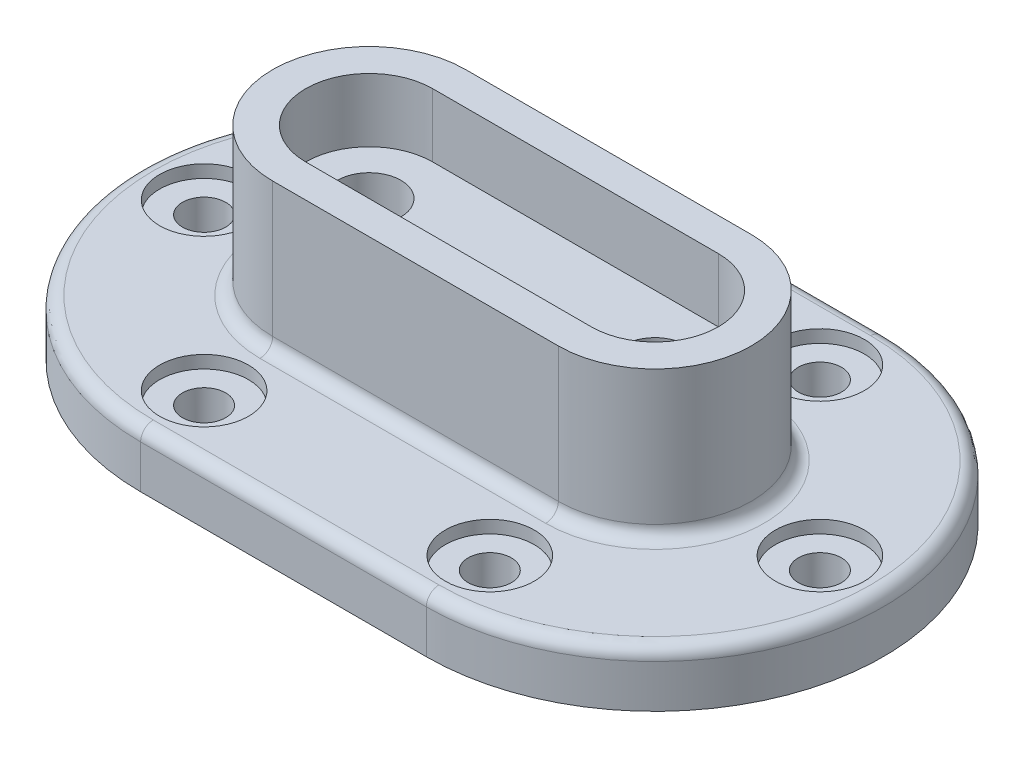
ISO-10303-21;
HEADER;
FILE_DESCRIPTION(('STEP AP214'),'2;1');
FILE_NAME('part.step','',(''),(''),'','','');
FILE_SCHEMA(('AUTOMOTIVE_DESIGN { 1 0 10303 214 1 1 1 1 }'));
ENDSEC;
DATA;
#1=APPLICATION_CONTEXT('core data for automotive mechanical design processes');
#2=APPLICATION_PROTOCOL_DEFINITION('international standard','automotive_design',2000,#1);
#3=PRODUCT_CONTEXT('',#1,'mechanical');
#4=PRODUCT('Part','Part','',(#3));
#5=PRODUCT_RELATED_PRODUCT_CATEGORY('part','',(#4));
#6=PRODUCT_DEFINITION_FORMATION('','',#4);
#7=PRODUCT_DEFINITION_CONTEXT('part definition',#1,'design');
#8=PRODUCT_DEFINITION('design','',#6,#7);
#9=PRODUCT_DEFINITION_SHAPE('','',#8);
#10=(LENGTH_UNIT() NAMED_UNIT(*) SI_UNIT(.MILLI.,.METRE.));
#11=(NAMED_UNIT(*) PLANE_ANGLE_UNIT() SI_UNIT($,.RADIAN.));
#12=(NAMED_UNIT(*) SI_UNIT($,.STERADIAN.) SOLID_ANGLE_UNIT());
#13=UNCERTAINTY_MEASURE_WITH_UNIT(LENGTH_MEASURE(1.E-05),#10,'distance_accuracy_value','');
#14=(GEOMETRIC_REPRESENTATION_CONTEXT(3) GLOBAL_UNCERTAINTY_ASSIGNED_CONTEXT((#13)) GLOBAL_UNIT_ASSIGNED_CONTEXT((#10,
#11,#12)) REPRESENTATION_CONTEXT('',''));
#15=CARTESIAN_POINT('',(0.,0.,0.));
#16=DIRECTION('',(0.,0.,1.));
#17=DIRECTION('',(1.,0.,0.));
#18=AXIS2_PLACEMENT_3D('',#15,#16,#17);
#19=CARTESIAN_POINT('',(11.25,4.4,0.));
#20=DIRECTION('',(0.,-1.,0.));
#21=DIRECTION('',(0.,0.,-1.));
#22=AXIS2_PLACEMENT_3D('',#19,#20,#21);
#23=CYLINDRICAL_SURFACE('',#22,18.);
#24=DIRECTION('',(0.,-1.,0.));
#25=VECTOR('',#24,1.);
#26=CARTESIAN_POINT('',(11.25,4.4,-18.));
#27=LINE('',#26,#25);
#28=CARTESIAN_POINT('',(11.25,3.4,-18.));
#29=VERTEX_POINT('',#28);
#30=CARTESIAN_POINT('',(11.25,0.,-18.));
#31=VERTEX_POINT('',#30);
#32=EDGE_CURVE('E243',#29,#31,#27,.T.);
#33=ORIENTED_EDGE('',*,*,#32,.F.);
#34=CARTESIAN_POINT('',(11.25,3.4,0.));
#35=DIRECTION('',(0.,1.,0.));
#36=DIRECTION('',(0.,0.,1.));
#37=AXIS2_PLACEMENT_3D('',#34,#35,#36);
#38=CIRCLE('',#37,18.);
#39=CARTESIAN_POINT('',(11.25,3.4,18.));
#40=VERTEX_POINT('',#39);
#41=EDGE_CURVE('E68',#29,#40,#38,.F.);
#42=ORIENTED_EDGE('',*,*,#41,.T.);
#43=DIRECTION('',(0.,-1.,0.));
#44=VECTOR('',#43,1.);
#45=CARTESIAN_POINT('',(11.25,4.4,18.));
#46=LINE('',#45,#44);
#47=CARTESIAN_POINT('',(11.25,0.,18.));
#48=VERTEX_POINT('',#47);
#49=EDGE_CURVE('E232',#40,#48,#46,.T.);
#50=ORIENTED_EDGE('',*,*,#49,.T.);
#51=CARTESIAN_POINT('',(11.25,0.,0.));
#52=DIRECTION('',(0.,1.,0.));
#53=DIRECTION('',(0.,0.,1.));
#54=AXIS2_PLACEMENT_3D('',#51,#52,#53);
#55=CIRCLE('',#54,18.);
#56=EDGE_CURVE('E224',#48,#31,#55,.T.);
#57=ORIENTED_EDGE('',*,*,#56,.T.);
#58=EDGE_LOOP('',(#33,#42,#50,#57));
#59=FACE_BOUND('',#58,.T.);
#60=ADVANCED_FACE('F41',(#59),#23,.T.);
#61=CARTESIAN_POINT('',(11.25,4.4,-18.));
#62=DIRECTION('',(0.,0.,1.));
#63=DIRECTION('',(1.,0.,0.));
#64=AXIS2_PLACEMENT_3D('',#61,#62,#63);
#65=PLANE('',#64);
#66=DIRECTION('',(0.,-1.,0.));
#67=VECTOR('',#66,1.);
#68=CARTESIAN_POINT('',(-11.25,4.4,-18.));
#69=LINE('',#68,#67);
#70=CARTESIAN_POINT('',(-11.25,3.4,-18.));
#71=VERTEX_POINT('',#70);
#72=CARTESIAN_POINT('',(-11.25,0.,-18.));
#73=VERTEX_POINT('',#72);
#74=EDGE_CURVE('E239',#71,#73,#69,.T.);
#75=ORIENTED_EDGE('',*,*,#74,.F.);
#76=DIRECTION('',(-1.,0.,0.));
#77=VECTOR('',#76,1.);
#78=CARTESIAN_POINT('',(11.25,3.4,-18.));
#79=LINE('',#78,#77);
#80=EDGE_CURVE('E286',#71,#29,#79,.F.);
#81=ORIENTED_EDGE('',*,*,#80,.T.);
#82=ORIENTED_EDGE('',*,*,#32,.T.);
#83=DIRECTION('',(-1.,0.,0.));
#84=VECTOR('',#83,1.);
#85=CARTESIAN_POINT('',(11.25,0.,-18.));
#86=LINE('',#85,#84);
#87=EDGE_CURVE('E228',#31,#73,#86,.T.);
#88=ORIENTED_EDGE('',*,*,#87,.T.);
#89=EDGE_LOOP('',(#75,#81,#82,#88));
#90=FACE_BOUND('',#89,.T.);
#91=ADVANCED_FACE('F328',(#90),#65,.F.);
#92=CARTESIAN_POINT('',(-11.25,4.4,0.));
#93=DIRECTION('',(0.,-1.,0.));
#94=DIRECTION('',(0.,0.,-1.));
#95=AXIS2_PLACEMENT_3D('',#92,#93,#94);
#96=CYLINDRICAL_SURFACE('',#95,18.);
#97=DIRECTION('',(0.,-1.,0.));
#98=VECTOR('',#97,1.);
#99=CARTESIAN_POINT('',(-11.25,4.4,18.));
#100=LINE('',#99,#98);
#101=CARTESIAN_POINT('',(-11.25,3.4,18.));
#102=VERTEX_POINT('',#101);
#103=CARTESIAN_POINT('',(-11.25,0.,18.));
#104=VERTEX_POINT('',#103);
#105=EDGE_CURVE('E240',#102,#104,#100,.T.);
#106=ORIENTED_EDGE('',*,*,#105,.F.);
#107=CARTESIAN_POINT('',(-11.25,3.4,0.));
#108=DIRECTION('',(0.,1.,0.));
#109=DIRECTION('',(0.,0.,1.));
#110=AXIS2_PLACEMENT_3D('',#107,#108,#109);
#111=CIRCLE('',#110,18.);
#112=EDGE_CURVE('E11',#102,#71,#111,.F.);
#113=ORIENTED_EDGE('',*,*,#112,.T.);
#114=ORIENTED_EDGE('',*,*,#74,.T.);
#115=CARTESIAN_POINT('',(-11.25,0.,0.));
#116=DIRECTION('',(0.,1.,0.));
#117=DIRECTION('',(0.,0.,1.));
#118=AXIS2_PLACEMENT_3D('',#115,#116,#117);
#119=CIRCLE('',#118,18.);
#120=EDGE_CURVE('E227',#73,#104,#119,.T.);
#121=ORIENTED_EDGE('',*,*,#120,.T.);
#122=EDGE_LOOP('',(#106,#113,#114,#121));
#123=FACE_BOUND('',#122,.T.);
#124=ADVANCED_FACE('F326',(#123),#96,.T.);
#125=CARTESIAN_POINT('',(11.25,4.4,18.));
#126=DIRECTION('',(0.,0.,-1.));
#127=DIRECTION('',(-1.,0.,0.));
#128=AXIS2_PLACEMENT_3D('',#125,#126,#127);
#129=PLANE('',#128);
#130=ORIENTED_EDGE('',*,*,#49,.F.);
#131=DIRECTION('',(1.,0.,0.));
#132=VECTOR('',#131,1.);
#133=CARTESIAN_POINT('',(-11.25,3.4,18.));
#134=LINE('',#133,#132);
#135=EDGE_CURVE('E59',#40,#102,#134,.F.);
#136=ORIENTED_EDGE('',*,*,#135,.T.);
#137=ORIENTED_EDGE('',*,*,#105,.T.);
#138=DIRECTION('',(1.,0.,0.));
#139=VECTOR('',#138,1.);
#140=CARTESIAN_POINT('',(11.25,0.,18.));
#141=LINE('',#140,#139);
#142=EDGE_CURVE('E235',#104,#48,#141,.T.);
#143=ORIENTED_EDGE('',*,*,#142,.T.);
#144=EDGE_LOOP('',(#130,#136,#137,#143));
#145=FACE_BOUND('',#144,.T.);
#146=ADVANCED_FACE('F339',(#145),#129,.F.);
#147=CARTESIAN_POINT('',(11.25,4.4,0.));
#148=DIRECTION('',(0.,1.,0.));
#149=DIRECTION('',(0.,0.,1.));
#150=AXIS2_PLACEMENT_3D('',#147,#148,#149);
#151=PLANE('',#150);
#152=CARTESIAN_POINT('',(-11.25,4.4,0.));
#153=DIRECTION('',(0.,1.,0.));
#154=DIRECTION('',(0.,0.,1.));
#155=AXIS2_PLACEMENT_3D('',#152,#153,#154);
#156=CIRCLE('',#155,8.6);
#157=CARTESIAN_POINT('',(-11.25,4.4,8.6));
#158=VERTEX_POINT('',#157);
#159=CARTESIAN_POINT('',(-11.25,4.4,-8.6));
#160=VERTEX_POINT('',#159);
#161=EDGE_CURVE('E274',#158,#160,#156,.F.);
#162=ORIENTED_EDGE('',*,*,#161,.T.);
#163=DIRECTION('',(-1.,0.,0.));
#164=VECTOR('',#163,1.);
#165=CARTESIAN_POINT('',(11.25,4.4,-8.6));
#166=LINE('',#165,#164);
#167=CARTESIAN_POINT('',(11.25,4.4,-8.6));
#168=VERTEX_POINT('',#167);
#169=EDGE_CURVE('E283',#160,#168,#166,.F.);
#170=ORIENTED_EDGE('',*,*,#169,.T.);
#171=CARTESIAN_POINT('',(11.25,4.4,0.));
#172=DIRECTION('',(0.,1.,0.));
#173=DIRECTION('',(0.,0.,1.));
#174=AXIS2_PLACEMENT_3D('',#171,#172,#173);
#175=CIRCLE('',#174,8.6);
#176=CARTESIAN_POINT('',(11.25,4.4,8.6));
#177=VERTEX_POINT('',#176);
#178=EDGE_CURVE('E276',#168,#177,#175,.F.);
#179=ORIENTED_EDGE('',*,*,#178,.T.);
#180=DIRECTION('',(1.,0.,0.));
#181=VECTOR('',#180,1.);
#182=CARTESIAN_POINT('',(11.25,4.4,8.6));
#183=LINE('',#182,#181);
#184=EDGE_CURVE('E280',#177,#158,#183,.F.);
#185=ORIENTED_EDGE('',*,*,#184,.T.);
#186=EDGE_LOOP('',(#162,#170,#179,#185));
#187=FACE_BOUND('',#186,.T.);
#188=CARTESIAN_POINT('',(11.25,4.4,0.));
#189=DIRECTION('',(0.,1.,0.));
#190=DIRECTION('',(0.,0.,1.));
#191=AXIS2_PLACEMENT_3D('',#188,#189,#190);
#192=CIRCLE('',#191,17.);
#193=CARTESIAN_POINT('',(11.25,4.4,17.));
#194=VERTEX_POINT('',#193);
#195=CARTESIAN_POINT('',(11.25,4.4,-17.));
#196=VERTEX_POINT('',#195);
#197=EDGE_CURVE('E269',#194,#196,#192,.T.);
#198=ORIENTED_EDGE('',*,*,#197,.T.);
#199=DIRECTION('',(-1.,0.,0.));
#200=VECTOR('',#199,1.);
#201=CARTESIAN_POINT('',(-11.25,4.4,-17.));
#202=LINE('',#201,#200);
#203=CARTESIAN_POINT('',(-11.25,4.4,-17.));
#204=VERTEX_POINT('',#203);
#205=EDGE_CURVE('E275',#196,#204,#202,.T.);
#206=ORIENTED_EDGE('',*,*,#205,.T.);
#207=CARTESIAN_POINT('',(-11.25,4.4,0.));
#208=DIRECTION('',(0.,1.,0.));
#209=DIRECTION('',(0.,0.,1.));
#210=AXIS2_PLACEMENT_3D('',#207,#208,#209);
#211=CIRCLE('',#210,17.);
#212=CARTESIAN_POINT('',(-11.25,4.4,17.));
#213=VERTEX_POINT('',#212);
#214=EDGE_CURVE('E266',#204,#213,#211,.T.);
#215=ORIENTED_EDGE('',*,*,#214,.T.);
#216=DIRECTION('',(1.,0.,0.));
#217=VECTOR('',#216,1.);
#218=CARTESIAN_POINT('',(11.25,4.4,17.));
#219=LINE('',#218,#217);
#220=EDGE_CURVE('E268',#213,#194,#219,.T.);
#221=ORIENTED_EDGE('',*,*,#220,.T.);
#222=EDGE_LOOP('',(#198,#206,#215,#221));
#223=FACE_BOUND('',#222,.T.);
#224=CARTESIAN_POINT('',(24.2500000000001,4.4,-1.66533453693773E-13));
#225=DIRECTION('',(0.,1.,0.));
#226=DIRECTION('',(0.,0.,-1.));
#227=AXIS2_PLACEMENT_3D('',#224,#225,#226);
#228=CIRCLE('',#227,3.5);
#229=CARTESIAN_POINT('',(24.2500000000001,4.4,-3.50000000000017));
#230=VERTEX_POINT('',#229);
#231=EDGE_CURVE('E347',#230,#230,#228,.T.);
#232=ORIENTED_EDGE('',*,*,#231,.F.);
#233=EDGE_LOOP('',(#232));
#234=FACE_BOUND('',#233,.T.);
#235=CARTESIAN_POINT('',(-24.25,4.4,0.));
#236=DIRECTION('',(0.,1.,0.));
#237=DIRECTION('',(0.,0.,1.));
#238=AXIS2_PLACEMENT_3D('',#235,#236,#237);
#239=CIRCLE('',#238,3.5);
#240=CARTESIAN_POINT('',(-24.25,4.4,3.5));
#241=VERTEX_POINT('',#240);
#242=EDGE_CURVE('E348',#241,#241,#239,.T.);
#243=ORIENTED_EDGE('',*,*,#242,.F.);
#244=EDGE_LOOP('',(#243));
#245=FACE_BOUND('',#244,.T.);
#246=CARTESIAN_POINT('',(-11.25,4.4,13.));
#247=DIRECTION('',(0.,1.,0.));
#248=DIRECTION('',(0.,0.,-1.));
#249=AXIS2_PLACEMENT_3D('',#246,#247,#248);
#250=CIRCLE('',#249,3.5);
#251=CARTESIAN_POINT('',(-11.25,4.4,9.5));
#252=VERTEX_POINT('',#251);
#253=EDGE_CURVE('E352',#252,#252,#250,.T.);
#254=ORIENTED_EDGE('',*,*,#253,.F.);
#255=EDGE_LOOP('',(#254));
#256=FACE_BOUND('',#255,.T.);
#257=CARTESIAN_POINT('',(11.25,4.4,13.));
#258=DIRECTION('',(0.,1.,0.));
#259=DIRECTION('',(0.,0.,1.));
#260=AXIS2_PLACEMENT_3D('',#257,#258,#259);
#261=CIRCLE('',#260,3.5);
#262=CARTESIAN_POINT('',(11.25,4.4,16.5));
#263=VERTEX_POINT('',#262);
#264=EDGE_CURVE('E356',#263,#263,#261,.T.);
#265=ORIENTED_EDGE('',*,*,#264,.F.);
#266=EDGE_LOOP('',(#265));
#267=FACE_BOUND('',#266,.T.);
#268=CARTESIAN_POINT('',(11.25,4.4,-13.));
#269=DIRECTION('',(0.,1.,0.));
#270=DIRECTION('',(0.,0.,-1.));
#271=AXIS2_PLACEMENT_3D('',#268,#269,#270);
#272=CIRCLE('',#271,3.5);
#273=CARTESIAN_POINT('',(11.25,4.4,-16.5));
#274=VERTEX_POINT('',#273);
#275=EDGE_CURVE('E362',#274,#274,#272,.T.);
#276=ORIENTED_EDGE('',*,*,#275,.F.);
#277=EDGE_LOOP('',(#276));
#278=FACE_BOUND('',#277,.T.);
#279=CARTESIAN_POINT('',(-11.25,4.4,-13.));
#280=DIRECTION('',(0.,1.,0.));
#281=DIRECTION('',(0.,0.,1.));
#282=AXIS2_PLACEMENT_3D('',#279,#280,#281);
#283=CIRCLE('',#282,3.5);
#284=CARTESIAN_POINT('',(-11.25,4.4,-9.5));
#285=VERTEX_POINT('',#284);
#286=EDGE_CURVE('E188',#285,#285,#283,.T.);
#287=ORIENTED_EDGE('',*,*,#286,.F.);
#288=EDGE_LOOP('',(#287));
#289=FACE_BOUND('',#288,.T.);
#290=ADVANCED_FACE('F338',(#187,#223,#234,#245,#256,#267,#278,#289),#151,.T.);
#291=CARTESIAN_POINT('',(11.25,0.,0.));
#292=DIRECTION('',(0.,1.,0.));
#293=DIRECTION('',(0.,0.,1.));
#294=AXIS2_PLACEMENT_3D('',#291,#292,#293);
#295=PLANE('',#294);
#296=CARTESIAN_POINT('',(-11.25,0.,0.));
#297=DIRECTION('',(0.,1.,0.));
#298=DIRECTION('',(0.,0.,1.));
#299=AXIS2_PLACEMENT_3D('',#296,#297,#298);
#300=CIRCLE('',#299,2.5);
#301=CARTESIAN_POINT('',(-11.25,0.,2.5));
#302=VERTEX_POINT('',#301);
#303=EDGE_CURVE('E797',#302,#302,#300,.T.);
#304=ORIENTED_EDGE('',*,*,#303,.T.);
#305=EDGE_LOOP('',(#304));
#306=FACE_BOUND('',#305,.T.);
#307=CARTESIAN_POINT('',(11.25,0.,0.));
#308=DIRECTION('',(0.,1.,0.));
#309=DIRECTION('',(0.,0.,1.));
#310=AXIS2_PLACEMENT_3D('',#307,#308,#309);
#311=CIRCLE('',#310,2.5);
#312=CARTESIAN_POINT('',(11.25,0.,2.5));
#313=VERTEX_POINT('',#312);
#314=EDGE_CURVE('E802',#313,#313,#311,.T.);
#315=ORIENTED_EDGE('',*,*,#314,.T.);
#316=EDGE_LOOP('',(#315));
#317=FACE_BOUND('',#316,.T.);
#318=CARTESIAN_POINT('',(24.25,0.,0.));
#319=DIRECTION('',(0.,1.,0.));
#320=DIRECTION('',(0.,0.,1.));
#321=AXIS2_PLACEMENT_3D('',#318,#319,#320);
#322=CIRCLE('',#321,1.7);
#323=CARTESIAN_POINT('',(24.25,0.,1.7));
#324=VERTEX_POINT('',#323);
#325=EDGE_CURVE('E257',#324,#324,#322,.T.);
#326=ORIENTED_EDGE('',*,*,#325,.T.);
#327=EDGE_LOOP('',(#326));
#328=FACE_BOUND('',#327,.T.);
#329=CARTESIAN_POINT('',(-24.25,0.,0.));
#330=DIRECTION('',(0.,1.,0.));
#331=DIRECTION('',(0.,0.,1.));
#332=AXIS2_PLACEMENT_3D('',#329,#330,#331);
#333=CIRCLE('',#332,1.7);
#334=CARTESIAN_POINT('',(-24.25,0.,1.7));
#335=VERTEX_POINT('',#334);
#336=EDGE_CURVE('E260',#335,#335,#333,.T.);
#337=ORIENTED_EDGE('',*,*,#336,.T.);
#338=EDGE_LOOP('',(#337));
#339=FACE_BOUND('',#338,.T.);
#340=CARTESIAN_POINT('',(-11.25,0.,13.));
#341=DIRECTION('',(0.,1.,0.));
#342=DIRECTION('',(0.,0.,1.));
#343=AXIS2_PLACEMENT_3D('',#340,#341,#342);
#344=CIRCLE('',#343,1.7);
#345=CARTESIAN_POINT('',(-11.25,0.,14.7));
#346=VERTEX_POINT('',#345);
#347=EDGE_CURVE('E255',#346,#346,#344,.T.);
#348=ORIENTED_EDGE('',*,*,#347,.T.);
#349=EDGE_LOOP('',(#348));
#350=FACE_BOUND('',#349,.T.);
#351=CARTESIAN_POINT('',(11.25,0.,13.));
#352=DIRECTION('',(0.,1.,0.));
#353=DIRECTION('',(0.,0.,1.));
#354=AXIS2_PLACEMENT_3D('',#351,#352,#353);
#355=CIRCLE('',#354,1.7);
#356=CARTESIAN_POINT('',(11.25,0.,14.7));
#357=VERTEX_POINT('',#356);
#358=EDGE_CURVE('E253',#357,#357,#355,.T.);
#359=ORIENTED_EDGE('',*,*,#358,.T.);
#360=EDGE_LOOP('',(#359));
#361=FACE_BOUND('',#360,.T.);
#362=CARTESIAN_POINT('',(11.25,0.,-13.));
#363=DIRECTION('',(0.,1.,0.));
#364=DIRECTION('',(0.,0.,1.));
#365=AXIS2_PLACEMENT_3D('',#362,#363,#364);
#366=CIRCLE('',#365,1.7);
#367=CARTESIAN_POINT('',(11.25,0.,-11.3));
#368=VERTEX_POINT('',#367);
#369=EDGE_CURVE('E250',#368,#368,#366,.T.);
#370=ORIENTED_EDGE('',*,*,#369,.T.);
#371=EDGE_LOOP('',(#370));
#372=FACE_BOUND('',#371,.T.);
#373=CARTESIAN_POINT('',(-11.25,0.,-13.));
#374=DIRECTION('',(0.,1.,0.));
#375=DIRECTION('',(0.,0.,1.));
#376=AXIS2_PLACEMENT_3D('',#373,#374,#375);
#377=CIRCLE('',#376,1.7);
#378=CARTESIAN_POINT('',(-11.25,0.,-11.3));
#379=VERTEX_POINT('',#378);
#380=EDGE_CURVE('E242',#379,#379,#377,.T.);
#381=ORIENTED_EDGE('',*,*,#380,.T.);
#382=EDGE_LOOP('',(#381));
#383=FACE_BOUND('',#382,.T.);
#384=ORIENTED_EDGE('',*,*,#56,.F.);
#385=ORIENTED_EDGE('',*,*,#142,.F.);
#386=ORIENTED_EDGE('',*,*,#120,.F.);
#387=ORIENTED_EDGE('',*,*,#87,.F.);
#388=EDGE_LOOP('',(#384,#385,#386,#387));
#389=FACE_BOUND('',#388,.T.);
#390=ADVANCED_FACE('F337',(#306,#317,#328,#339,#350,#361,#372,#383,#389),#295,.F.);
#391=CARTESIAN_POINT('',(-11.25,16.,0.));
#392=DIRECTION('',(0.,-1.,0.));
#393=DIRECTION('',(0.,0.,-1.));
#394=AXIS2_PLACEMENT_3D('',#391,#392,#393);
#395=CYLINDRICAL_SURFACE('',#394,7.6);
#396=DIRECTION('',(0.,-1.,0.));
#397=VECTOR('',#396,1.);
#398=CARTESIAN_POINT('',(-11.25,16.,-7.6));
#399=LINE('',#398,#397);
#400=CARTESIAN_POINT('',(-11.25,16.,-7.6));
#401=VERTEX_POINT('',#400);
#402=CARTESIAN_POINT('',(-11.25,5.4,-7.6));
#403=VERTEX_POINT('',#402);
#404=EDGE_CURVE('E211',#401,#403,#399,.T.);
#405=ORIENTED_EDGE('',*,*,#404,.T.);
#406=CARTESIAN_POINT('',(-11.25,5.4,0.));
#407=DIRECTION('',(0.,1.,0.));
#408=DIRECTION('',(0.,0.,1.));
#409=AXIS2_PLACEMENT_3D('',#406,#407,#408);
#410=CIRCLE('',#409,7.6);
#411=CARTESIAN_POINT('',(-11.25,5.4,7.6));
#412=VERTEX_POINT('',#411);
#413=EDGE_CURVE('E49',#403,#412,#410,.T.);
#414=ORIENTED_EDGE('',*,*,#413,.T.);
#415=DIRECTION('',(0.,-1.,0.));
#416=VECTOR('',#415,1.);
#417=CARTESIAN_POINT('',(-11.25,16.,7.6));
#418=LINE('',#417,#416);
#419=CARTESIAN_POINT('',(-11.25,16.,7.6));
#420=VERTEX_POINT('',#419);
#421=EDGE_CURVE('E219',#420,#412,#418,.T.);
#422=ORIENTED_EDGE('',*,*,#421,.F.);
#423=CARTESIAN_POINT('',(-11.25,16.,0.));
#424=DIRECTION('',(0.,1.,0.));
#425=DIRECTION('',(0.,0.,1.));
#426=AXIS2_PLACEMENT_3D('',#423,#424,#425);
#427=CIRCLE('',#426,7.6);
#428=EDGE_CURVE('E200',#401,#420,#427,.T.);
#429=ORIENTED_EDGE('',*,*,#428,.F.);
#430=EDGE_LOOP('',(#405,#414,#422,#429));
#431=FACE_BOUND('',#430,.T.);
#432=ADVANCED_FACE('F493',(#431),#395,.T.);
#433=CARTESIAN_POINT('',(-11.25,16.,7.6));
#434=DIRECTION('',(0.,0.,-1.));
#435=DIRECTION('',(-1.,0.,0.));
#436=AXIS2_PLACEMENT_3D('',#433,#434,#435);
#437=PLANE('',#436);
#438=ORIENTED_EDGE('',*,*,#421,.T.);
#439=DIRECTION('',(1.,0.,0.));
#440=VECTOR('',#439,1.);
#441=CARTESIAN_POINT('',(-11.25,5.4,7.6));
#442=LINE('',#441,#440);
#443=CARTESIAN_POINT('',(11.25,5.4,7.6));
#444=VERTEX_POINT('',#443);
#445=EDGE_CURVE('E288',#412,#444,#442,.T.);
#446=ORIENTED_EDGE('',*,*,#445,.T.);
#447=DIRECTION('',(0.,-1.,0.));
#448=VECTOR('',#447,1.);
#449=CARTESIAN_POINT('',(11.25,16.,7.6));
#450=LINE('',#449,#448);
#451=CARTESIAN_POINT('',(11.25,16.,7.6));
#452=VERTEX_POINT('',#451);
#453=EDGE_CURVE('E220',#452,#444,#450,.T.);
#454=ORIENTED_EDGE('',*,*,#453,.F.);
#455=DIRECTION('',(1.,0.,0.));
#456=VECTOR('',#455,1.);
#457=CARTESIAN_POINT('',(-11.25,16.,7.6));
#458=LINE('',#457,#456);
#459=EDGE_CURVE('E202',#420,#452,#458,.T.);
#460=ORIENTED_EDGE('',*,*,#459,.F.);
#461=EDGE_LOOP('',(#438,#446,#454,#460));
#462=FACE_BOUND('',#461,.T.);
#463=ADVANCED_FACE('F484',(#462),#437,.F.);
#464=CARTESIAN_POINT('',(11.25,16.,0.));
#465=DIRECTION('',(0.,-1.,0.));
#466=DIRECTION('',(0.,0.,-1.));
#467=AXIS2_PLACEMENT_3D('',#464,#465,#466);
#468=CYLINDRICAL_SURFACE('',#467,7.6);
#469=ORIENTED_EDGE('',*,*,#453,.T.);
#470=CARTESIAN_POINT('',(11.25,5.4,0.));
#471=DIRECTION('',(0.,1.,0.));
#472=DIRECTION('',(0.,0.,1.));
#473=AXIS2_PLACEMENT_3D('',#470,#471,#472);
#474=CIRCLE('',#473,7.6);
#475=CARTESIAN_POINT('',(11.25,5.4,-7.6));
#476=VERTEX_POINT('',#475);
#477=EDGE_CURVE('E282',#444,#476,#474,.T.);
#478=ORIENTED_EDGE('',*,*,#477,.T.);
#479=DIRECTION('',(0.,-1.,0.));
#480=VECTOR('',#479,1.);
#481=CARTESIAN_POINT('',(11.25,16.,-7.6));
#482=LINE('',#481,#480);
#483=CARTESIAN_POINT('',(11.25,16.,-7.6));
#484=VERTEX_POINT('',#483);
#485=EDGE_CURVE('E212',#484,#476,#482,.T.);
#486=ORIENTED_EDGE('',*,*,#485,.F.);
#487=CARTESIAN_POINT('',(11.25,16.,0.));
#488=DIRECTION('',(0.,1.,0.));
#489=DIRECTION('',(0.,0.,1.));
#490=AXIS2_PLACEMENT_3D('',#487,#488,#489);
#491=CIRCLE('',#490,7.6);
#492=EDGE_CURVE('E210',#452,#484,#491,.T.);
#493=ORIENTED_EDGE('',*,*,#492,.F.);
#494=EDGE_LOOP('',(#469,#478,#486,#493));
#495=FACE_BOUND('',#494,.T.);
#496=ADVANCED_FACE('F474',(#495),#468,.T.);
#497=CARTESIAN_POINT('',(-11.25,16.,-7.6));
#498=DIRECTION('',(0.,0.,1.));
#499=DIRECTION('',(1.,0.,0.));
#500=AXIS2_PLACEMENT_3D('',#497,#498,#499);
#501=PLANE('',#500);
#502=ORIENTED_EDGE('',*,*,#485,.T.);
#503=DIRECTION('',(-1.,0.,0.));
#504=VECTOR('',#503,1.);
#505=CARTESIAN_POINT('',(-11.25,5.4,-7.6));
#506=LINE('',#505,#504);
#507=EDGE_CURVE('E241',#476,#403,#506,.T.);
#508=ORIENTED_EDGE('',*,*,#507,.T.);
#509=ORIENTED_EDGE('',*,*,#404,.F.);
#510=DIRECTION('',(-1.,0.,0.));
#511=VECTOR('',#510,1.);
#512=CARTESIAN_POINT('',(-11.25,16.,-7.6));
#513=LINE('',#512,#511);
#514=EDGE_CURVE('E207',#484,#401,#513,.T.);
#515=ORIENTED_EDGE('',*,*,#514,.F.);
#516=EDGE_LOOP('',(#502,#508,#509,#515));
#517=FACE_BOUND('',#516,.T.);
#518=ADVANCED_FACE('F467',(#517),#501,.F.);
#519=CARTESIAN_POINT('',(-11.25,16.,0.));
#520=DIRECTION('',(0.,1.,0.));
#521=DIRECTION('',(0.,0.,1.));
#522=AXIS2_PLACEMENT_3D('',#519,#520,#521);
#523=PLANE('',#522);
#524=CARTESIAN_POINT('',(-11.25,16.,0.));
#525=DIRECTION('',(0.,1.,0.));
#526=DIRECTION('',(0.,0.,1.));
#527=AXIS2_PLACEMENT_3D('',#524,#525,#526);
#528=CIRCLE('',#527,5.);
#529=CARTESIAN_POINT('',(-11.25,16.,-5.));
#530=VERTEX_POINT('',#529);
#531=CARTESIAN_POINT('',(-11.25,16.,5.));
#532=VERTEX_POINT('',#531);
#533=EDGE_CURVE('E162',#530,#532,#528,.T.);
#534=ORIENTED_EDGE('',*,*,#533,.F.);
#535=DIRECTION('',(-1.,0.,0.));
#536=VECTOR('',#535,1.);
#537=CARTESIAN_POINT('',(-11.25,16.,-5.));
#538=LINE('',#537,#536);
#539=CARTESIAN_POINT('',(11.25,16.,-5.00000000000001));
#540=VERTEX_POINT('',#539);
#541=EDGE_CURVE('E177',#540,#530,#538,.T.);
#542=ORIENTED_EDGE('',*,*,#541,.F.);
#543=CARTESIAN_POINT('',(11.25,16.,0.));
#544=DIRECTION('',(0.,1.,0.));
#545=DIRECTION('',(0.,0.,1.));
#546=AXIS2_PLACEMENT_3D('',#543,#544,#545);
#547=CIRCLE('',#546,5.);
#548=CARTESIAN_POINT('',(11.25,16.,5.));
#549=VERTEX_POINT('',#548);
#550=EDGE_CURVE('E181',#549,#540,#547,.T.);
#551=ORIENTED_EDGE('',*,*,#550,.F.);
#552=DIRECTION('',(1.,0.,0.));
#553=VECTOR('',#552,1.);
#554=CARTESIAN_POINT('',(-11.25,16.,5.));
#555=LINE('',#554,#553);
#556=EDGE_CURVE('E195',#532,#549,#555,.T.);
#557=ORIENTED_EDGE('',*,*,#556,.F.);
#558=EDGE_LOOP('',(#534,#542,#551,#557));
#559=FACE_BOUND('',#558,.T.);
#560=ORIENTED_EDGE('',*,*,#428,.T.);
#561=ORIENTED_EDGE('',*,*,#459,.T.);
#562=ORIENTED_EDGE('',*,*,#492,.T.);
#563=ORIENTED_EDGE('',*,*,#514,.T.);
#564=EDGE_LOOP('',(#560,#561,#562,#563));
#565=FACE_BOUND('',#564,.T.);
#566=ADVANCED_FACE('F475',(#559,#565),#523,.T.);
#567=CARTESIAN_POINT('',(-11.25,11.,0.));
#568=DIRECTION('',(0.,1.,0.));
#569=DIRECTION('',(0.,0.,1.));
#570=AXIS2_PLACEMENT_3D('',#567,#568,#569);
#571=CYLINDRICAL_SURFACE('',#570,5.);
#572=ORIENTED_EDGE('',*,*,#533,.T.);
#573=DIRECTION('',(0.,1.,0.));
#574=VECTOR('',#573,1.);
#575=CARTESIAN_POINT('',(-11.25,11.,5.));
#576=LINE('',#575,#574);
#577=CARTESIAN_POINT('',(-11.25,11.,5.));
#578=VERTEX_POINT('',#577);
#579=EDGE_CURVE('E156',#578,#532,#576,.T.);
#580=ORIENTED_EDGE('',*,*,#579,.F.);
#581=CARTESIAN_POINT('',(-11.25,11.,0.));
#582=DIRECTION('',(0.,1.,0.));
#583=DIRECTION('',(0.,0.,1.));
#584=AXIS2_PLACEMENT_3D('',#581,#582,#583);
#585=CIRCLE('',#584,5.);
#586=CARTESIAN_POINT('',(-11.25,11.,-5.));
#587=VERTEX_POINT('',#586);
#588=EDGE_CURVE('E159',#587,#578,#585,.T.);
#589=ORIENTED_EDGE('',*,*,#588,.F.);
#590=DIRECTION('',(0.,1.,0.));
#591=VECTOR('',#590,1.);
#592=CARTESIAN_POINT('',(-11.25,11.,-5.));
#593=LINE('',#592,#591);
#594=EDGE_CURVE('E197',#587,#530,#593,.T.);
#595=ORIENTED_EDGE('',*,*,#594,.T.);
#596=EDGE_LOOP('',(#572,#580,#589,#595));
#597=FACE_BOUND('',#596,.T.);
#598=ADVANCED_FACE('F158',(#597),#571,.F.);
#599=CARTESIAN_POINT('',(-11.25,11.,-5.));
#600=DIRECTION('',(0.,0.,-1.));
#601=DIRECTION('',(-1.,0.,0.));
#602=AXIS2_PLACEMENT_3D('',#599,#600,#601);
#603=PLANE('',#602);
#604=ORIENTED_EDGE('',*,*,#541,.T.);
#605=ORIENTED_EDGE('',*,*,#594,.F.);
#606=DIRECTION('',(-1.,0.,0.));
#607=VECTOR('',#606,1.);
#608=CARTESIAN_POINT('',(-11.25,11.,-5.));
#609=LINE('',#608,#607);
#610=CARTESIAN_POINT('',(11.25,11.,-5.00000000000001));
#611=VERTEX_POINT('',#610);
#612=EDGE_CURVE('E169',#611,#587,#609,.T.);
#613=ORIENTED_EDGE('',*,*,#612,.F.);
#614=DIRECTION('',(0.,1.,0.));
#615=VECTOR('',#614,1.);
#616=CARTESIAN_POINT('',(11.25,11.,-5.00000000000001));
#617=LINE('',#616,#615);
#618=EDGE_CURVE('E199',#611,#540,#617,.T.);
#619=ORIENTED_EDGE('',*,*,#618,.T.);
#620=EDGE_LOOP('',(#604,#605,#613,#619));
#621=FACE_BOUND('',#620,.T.);
#622=ADVANCED_FACE('F565',(#621),#603,.F.);
#623=CARTESIAN_POINT('',(11.25,11.,0.));
#624=DIRECTION('',(0.,1.,0.));
#625=DIRECTION('',(0.,0.,1.));
#626=AXIS2_PLACEMENT_3D('',#623,#624,#625);
#627=CYLINDRICAL_SURFACE('',#626,5.);
#628=ORIENTED_EDGE('',*,*,#550,.T.);
#629=ORIENTED_EDGE('',*,*,#618,.F.);
#630=CARTESIAN_POINT('',(11.25,11.,0.));
#631=DIRECTION('',(0.,1.,0.));
#632=DIRECTION('',(0.,0.,1.));
#633=AXIS2_PLACEMENT_3D('',#630,#631,#632);
#634=CIRCLE('',#633,5.);
#635=CARTESIAN_POINT('',(11.25,11.,5.));
#636=VERTEX_POINT('',#635);
#637=EDGE_CURVE('E178',#636,#611,#634,.T.);
#638=ORIENTED_EDGE('',*,*,#637,.F.);
#639=DIRECTION('',(0.,1.,0.));
#640=VECTOR('',#639,1.);
#641=CARTESIAN_POINT('',(11.25,11.,5.));
#642=LINE('',#641,#640);
#643=EDGE_CURVE('E170',#636,#549,#642,.T.);
#644=ORIENTED_EDGE('',*,*,#643,.T.);
#645=EDGE_LOOP('',(#628,#629,#638,#644));
#646=FACE_BOUND('',#645,.T.);
#647=ADVANCED_FACE('F568',(#646),#627,.F.);
#648=CARTESIAN_POINT('',(-11.25,11.,5.));
#649=DIRECTION('',(0.,0.,1.));
#650=DIRECTION('',(1.,0.,0.));
#651=AXIS2_PLACEMENT_3D('',#648,#649,#650);
#652=PLANE('',#651);
#653=ORIENTED_EDGE('',*,*,#556,.T.);
#654=ORIENTED_EDGE('',*,*,#643,.F.);
#655=DIRECTION('',(1.,0.,0.));
#656=VECTOR('',#655,1.);
#657=CARTESIAN_POINT('',(-11.25,11.,5.));
#658=LINE('',#657,#656);
#659=EDGE_CURVE('E173',#578,#636,#658,.T.);
#660=ORIENTED_EDGE('',*,*,#659,.F.);
#661=ORIENTED_EDGE('',*,*,#579,.T.);
#662=EDGE_LOOP('',(#653,#654,#660,#661));
#663=FACE_BOUND('',#662,.T.);
#664=ADVANCED_FACE('F175',(#663),#652,.F.);
#665=CARTESIAN_POINT('',(-11.25,11.,0.));
#666=DIRECTION('',(0.,1.,0.));
#667=DIRECTION('',(0.,0.,1.));
#668=AXIS2_PLACEMENT_3D('',#665,#666,#667);
#669=PLANE('',#668);
#670=CARTESIAN_POINT('',(-11.25,11.,0.));
#671=DIRECTION('',(0.,1.,0.));
#672=DIRECTION('',(0.,0.,1.));
#673=AXIS2_PLACEMENT_3D('',#670,#671,#672);
#674=CIRCLE('',#673,2.5);
#675=CARTESIAN_POINT('',(-11.25,11.,2.5));
#676=VERTEX_POINT('',#675);
#677=EDGE_CURVE('E800',#676,#676,#674,.T.);
#678=ORIENTED_EDGE('',*,*,#677,.F.);
#679=EDGE_LOOP('',(#678));
#680=FACE_BOUND('',#679,.T.);
#681=CARTESIAN_POINT('',(11.25,11.,0.));
#682=DIRECTION('',(0.,1.,0.));
#683=DIRECTION('',(0.,0.,1.));
#684=AXIS2_PLACEMENT_3D('',#681,#682,#683);
#685=CIRCLE('',#684,2.5);
#686=CARTESIAN_POINT('',(11.25,11.,2.5));
#687=VERTEX_POINT('',#686);
#688=EDGE_CURVE('E304',#687,#687,#685,.T.);
#689=ORIENTED_EDGE('',*,*,#688,.F.);
#690=EDGE_LOOP('',(#689));
#691=FACE_BOUND('',#690,.T.);
#692=ORIENTED_EDGE('',*,*,#588,.T.);
#693=ORIENTED_EDGE('',*,*,#659,.T.);
#694=ORIENTED_EDGE('',*,*,#637,.T.);
#695=ORIENTED_EDGE('',*,*,#612,.T.);
#696=EDGE_LOOP('',(#692,#693,#694,#695));
#697=FACE_BOUND('',#696,.T.);
#698=ADVANCED_FACE('F176',(#680,#691,#697),#669,.T.);
#699=CARTESIAN_POINT('',(-11.25,3.4,-13.));
#700=DIRECTION('',(0.,1.,0.));
#701=DIRECTION('',(0.,0.,1.));
#702=AXIS2_PLACEMENT_3D('',#699,#700,#701);
#703=CYLINDRICAL_SURFACE('',#702,3.5);
#704=CARTESIAN_POINT('',(-11.25,3.4,-13.));
#705=DIRECTION('',(0.,1.,0.));
#706=DIRECTION('',(0.,0.,1.));
#707=AXIS2_PLACEMENT_3D('',#704,#705,#706);
#708=CIRCLE('',#707,3.5);
#709=CARTESIAN_POINT('',(-11.25,3.4,-9.5));
#710=VERTEX_POINT('',#709);
#711=EDGE_CURVE('E191',#710,#710,#708,.T.);
#712=ORIENTED_EDGE('',*,*,#711,.F.);
#713=EDGE_LOOP('',(#712));
#714=FACE_BOUND('',#713,.T.);
#715=ORIENTED_EDGE('',*,*,#286,.T.);
#716=EDGE_LOOP('',(#715));
#717=FACE_BOUND('',#716,.T.);
#718=ADVANCED_FACE('F592',(#714,#717),#703,.F.);
#719=CARTESIAN_POINT('',(-11.25,3.4,-13.));
#720=DIRECTION('',(0.,1.,0.));
#721=DIRECTION('',(0.,0.,1.));
#722=AXIS2_PLACEMENT_3D('',#719,#720,#721);
#723=PLANE('',#722);
#724=CARTESIAN_POINT('',(-11.25,3.4,-13.));
#725=DIRECTION('',(0.,1.,0.));
#726=DIRECTION('',(0.,0.,1.));
#727=AXIS2_PLACEMENT_3D('',#724,#725,#726);
#728=CIRCLE('',#727,1.7);
#729=CARTESIAN_POINT('',(-11.25,3.4,-11.3));
#730=VERTEX_POINT('',#729);
#731=EDGE_CURVE('E246',#730,#730,#728,.T.);
#732=ORIENTED_EDGE('',*,*,#731,.F.);
#733=EDGE_LOOP('',(#732));
#734=FACE_BOUND('',#733,.T.);
#735=ORIENTED_EDGE('',*,*,#711,.T.);
#736=EDGE_LOOP('',(#735));
#737=FACE_BOUND('',#736,.T.);
#738=ADVANCED_FACE('F602',(#734,#737),#723,.T.);
#739=CARTESIAN_POINT('',(11.25,3.4,-13.));
#740=DIRECTION('',(0.,1.,0.));
#741=DIRECTION('',(0.,0.,1.));
#742=AXIS2_PLACEMENT_3D('',#739,#740,#741);
#743=CYLINDRICAL_SURFACE('',#742,3.5);
#744=CARTESIAN_POINT('',(11.25,3.4,-13.));
#745=DIRECTION('',(0.,1.,0.));
#746=DIRECTION('',(0.,0.,-1.));
#747=AXIS2_PLACEMENT_3D('',#744,#745,#746);
#748=CIRCLE('',#747,3.5);
#749=CARTESIAN_POINT('',(11.25,3.4,-16.5));
#750=VERTEX_POINT('',#749);
#751=EDGE_CURVE('E370',#750,#750,#748,.T.);
#752=ORIENTED_EDGE('',*,*,#751,.F.);
#753=EDGE_LOOP('',(#752));
#754=FACE_BOUND('',#753,.T.);
#755=ORIENTED_EDGE('',*,*,#275,.T.);
#756=EDGE_LOOP('',(#755));
#757=FACE_BOUND('',#756,.T.);
#758=ADVANCED_FACE('F613',(#754,#757),#743,.F.);
#759=CARTESIAN_POINT('',(11.25,3.4,-13.));
#760=DIRECTION('',(0.,-1.,0.));
#761=DIRECTION('',(0.,0.,-1.));
#762=AXIS2_PLACEMENT_3D('',#759,#760,#761);
#763=PLANE('',#762);
#764=CARTESIAN_POINT('',(11.25,3.4,-13.));
#765=DIRECTION('',(0.,1.,0.));
#766=DIRECTION('',(0.,0.,-1.));
#767=AXIS2_PLACEMENT_3D('',#764,#765,#766);
#768=CIRCLE('',#767,1.7);
#769=CARTESIAN_POINT('',(11.25,3.4,-14.7));
#770=VERTEX_POINT('',#769);
#771=EDGE_CURVE('E807',#770,#770,#768,.T.);
#772=ORIENTED_EDGE('',*,*,#771,.F.);
#773=EDGE_LOOP('',(#772));
#774=FACE_BOUND('',#773,.T.);
#775=ORIENTED_EDGE('',*,*,#751,.T.);
#776=EDGE_LOOP('',(#775));
#777=FACE_BOUND('',#776,.T.);
#778=ADVANCED_FACE('F617',(#774,#777),#763,.F.);
#779=CARTESIAN_POINT('',(11.25,3.4,13.));
#780=DIRECTION('',(0.,1.,0.));
#781=DIRECTION('',(0.,0.,1.));
#782=AXIS2_PLACEMENT_3D('',#779,#780,#781);
#783=CYLINDRICAL_SURFACE('',#782,3.5);
#784=CARTESIAN_POINT('',(11.25,3.4,13.));
#785=DIRECTION('',(0.,1.,0.));
#786=DIRECTION('',(0.,0.,1.));
#787=AXIS2_PLACEMENT_3D('',#784,#785,#786);
#788=CIRCLE('',#787,3.5);
#789=CARTESIAN_POINT('',(11.25,3.4,16.5));
#790=VERTEX_POINT('',#789);
#791=EDGE_CURVE('E376',#790,#790,#788,.T.);
#792=ORIENTED_EDGE('',*,*,#791,.F.);
#793=EDGE_LOOP('',(#792));
#794=FACE_BOUND('',#793,.T.);
#795=ORIENTED_EDGE('',*,*,#264,.T.);
#796=EDGE_LOOP('',(#795));
#797=FACE_BOUND('',#796,.T.);
#798=ADVANCED_FACE('F627',(#794,#797),#783,.F.);
#799=CARTESIAN_POINT('',(11.25,3.4,13.));
#800=DIRECTION('',(0.,1.,0.));
#801=DIRECTION('',(0.,0.,1.));
#802=AXIS2_PLACEMENT_3D('',#799,#800,#801);
#803=PLANE('',#802);
#804=CARTESIAN_POINT('',(11.25,3.4,13.));
#805=DIRECTION('',(0.,1.,0.));
#806=DIRECTION('',(0.,0.,1.));
#807=AXIS2_PLACEMENT_3D('',#804,#805,#806);
#808=CIRCLE('',#807,1.7);
#809=CARTESIAN_POINT('',(11.25,3.4,14.7));
#810=VERTEX_POINT('',#809);
#811=EDGE_CURVE('E813',#810,#810,#808,.T.);
#812=ORIENTED_EDGE('',*,*,#811,.F.);
#813=EDGE_LOOP('',(#812));
#814=FACE_BOUND('',#813,.T.);
#815=ORIENTED_EDGE('',*,*,#791,.T.);
#816=EDGE_LOOP('',(#815));
#817=FACE_BOUND('',#816,.T.);
#818=ADVANCED_FACE('F636',(#814,#817),#803,.T.);
#819=CARTESIAN_POINT('',(-11.25,3.4,13.));
#820=DIRECTION('',(0.,1.,0.));
#821=DIRECTION('',(0.,0.,1.));
#822=AXIS2_PLACEMENT_3D('',#819,#820,#821);
#823=CYLINDRICAL_SURFACE('',#822,3.5);
#824=CARTESIAN_POINT('',(-11.25,3.4,13.));
#825=DIRECTION('',(0.,1.,0.));
#826=DIRECTION('',(0.,0.,-1.));
#827=AXIS2_PLACEMENT_3D('',#824,#825,#826);
#828=CIRCLE('',#827,3.5);
#829=CARTESIAN_POINT('',(-11.25,3.4,9.5));
#830=VERTEX_POINT('',#829);
#831=EDGE_CURVE('E379',#830,#830,#828,.T.);
#832=ORIENTED_EDGE('',*,*,#831,.F.);
#833=EDGE_LOOP('',(#832));
#834=FACE_BOUND('',#833,.T.);
#835=ORIENTED_EDGE('',*,*,#253,.T.);
#836=EDGE_LOOP('',(#835));
#837=FACE_BOUND('',#836,.T.);
#838=ADVANCED_FACE('F650',(#834,#837),#823,.F.);
#839=CARTESIAN_POINT('',(-11.25,3.4,13.));
#840=DIRECTION('',(0.,-1.,0.));
#841=DIRECTION('',(0.,0.,-1.));
#842=AXIS2_PLACEMENT_3D('',#839,#840,#841);
#843=PLANE('',#842);
#844=CARTESIAN_POINT('',(-11.25,3.4,13.));
#845=DIRECTION('',(0.,1.,0.));
#846=DIRECTION('',(0.,0.,-1.));
#847=AXIS2_PLACEMENT_3D('',#844,#845,#846);
#848=CIRCLE('',#847,1.7);
#849=CARTESIAN_POINT('',(-11.25,3.4,11.3));
#850=VERTEX_POINT('',#849);
#851=EDGE_CURVE('E816',#850,#850,#848,.T.);
#852=ORIENTED_EDGE('',*,*,#851,.F.);
#853=EDGE_LOOP('',(#852));
#854=FACE_BOUND('',#853,.T.);
#855=ORIENTED_EDGE('',*,*,#831,.T.);
#856=EDGE_LOOP('',(#855));
#857=FACE_BOUND('',#856,.T.);
#858=ADVANCED_FACE('F656',(#854,#857),#843,.F.);
#859=CARTESIAN_POINT('',(-24.25,3.4,0.));
#860=DIRECTION('',(0.,1.,0.));
#861=DIRECTION('',(0.,0.,1.));
#862=AXIS2_PLACEMENT_3D('',#859,#860,#861);
#863=CYLINDRICAL_SURFACE('',#862,3.5);
#864=CARTESIAN_POINT('',(-24.25,3.4,0.));
#865=DIRECTION('',(0.,1.,0.));
#866=DIRECTION('',(0.,0.,1.));
#867=AXIS2_PLACEMENT_3D('',#864,#865,#866);
#868=CIRCLE('',#867,3.5);
#869=CARTESIAN_POINT('',(-24.25,3.4,3.5));
#870=VERTEX_POINT('',#869);
#871=EDGE_CURVE('E383',#870,#870,#868,.T.);
#872=ORIENTED_EDGE('',*,*,#871,.F.);
#873=EDGE_LOOP('',(#872));
#874=FACE_BOUND('',#873,.T.);
#875=ORIENTED_EDGE('',*,*,#242,.T.);
#876=EDGE_LOOP('',(#875));
#877=FACE_BOUND('',#876,.T.);
#878=ADVANCED_FACE('F410',(#874,#877),#863,.F.);
#879=CARTESIAN_POINT('',(-24.25,3.4,0.));
#880=DIRECTION('',(0.,1.,0.));
#881=DIRECTION('',(0.,0.,1.));
#882=AXIS2_PLACEMENT_3D('',#879,#880,#881);
#883=PLANE('',#882);
#884=CARTESIAN_POINT('',(-24.25,3.4,0.));
#885=DIRECTION('',(0.,1.,0.));
#886=DIRECTION('',(0.,0.,1.));
#887=AXIS2_PLACEMENT_3D('',#884,#885,#886);
#888=CIRCLE('',#887,1.7);
#889=CARTESIAN_POINT('',(-24.25,3.4,1.7));
#890=VERTEX_POINT('',#889);
#891=EDGE_CURVE('E804',#890,#890,#888,.T.);
#892=ORIENTED_EDGE('',*,*,#891,.F.);
#893=EDGE_LOOP('',(#892));
#894=FACE_BOUND('',#893,.T.);
#895=ORIENTED_EDGE('',*,*,#871,.T.);
#896=EDGE_LOOP('',(#895));
#897=FACE_BOUND('',#896,.T.);
#898=ADVANCED_FACE('F398',(#894,#897),#883,.T.);
#899=CARTESIAN_POINT('',(24.2500000000001,3.4,-1.66533453693773E-13));
#900=DIRECTION('',(0.,1.,0.));
#901=DIRECTION('',(0.,0.,1.));
#902=AXIS2_PLACEMENT_3D('',#899,#900,#901);
#903=CYLINDRICAL_SURFACE('',#902,3.5);
#904=CARTESIAN_POINT('',(24.2500000000001,3.4,-1.66533453693773E-13));
#905=DIRECTION('',(0.,1.,0.));
#906=DIRECTION('',(0.,0.,-1.));
#907=AXIS2_PLACEMENT_3D('',#904,#905,#906);
#908=CIRCLE('',#907,3.5);
#909=CARTESIAN_POINT('',(24.2500000000001,3.4,-3.50000000000017));
#910=VERTEX_POINT('',#909);
#911=EDGE_CURVE('E263',#910,#910,#908,.T.);
#912=ORIENTED_EDGE('',*,*,#911,.F.);
#913=EDGE_LOOP('',(#912));
#914=FACE_BOUND('',#913,.T.);
#915=ORIENTED_EDGE('',*,*,#231,.T.);
#916=EDGE_LOOP('',(#915));
#917=FACE_BOUND('',#916,.T.);
#918=ADVANCED_FACE('F391',(#914,#917),#903,.F.);
#919=CARTESIAN_POINT('',(24.2500000000001,3.4,-1.66533453693773E-13));
#920=DIRECTION('',(0.,-1.,0.));
#921=DIRECTION('',(0.,0.,-1.));
#922=AXIS2_PLACEMENT_3D('',#919,#920,#921);
#923=PLANE('',#922);
#924=CARTESIAN_POINT('',(24.25,3.4,0.));
#925=DIRECTION('',(0.,1.,0.));
#926=DIRECTION('',(0.,0.,-1.));
#927=AXIS2_PLACEMENT_3D('',#924,#925,#926);
#928=CIRCLE('',#927,1.7);
#929=CARTESIAN_POINT('',(24.25,3.4,-1.7));
#930=VERTEX_POINT('',#929);
#931=EDGE_CURVE('E803',#930,#930,#928,.T.);
#932=ORIENTED_EDGE('',*,*,#931,.F.);
#933=EDGE_LOOP('',(#932));
#934=FACE_BOUND('',#933,.T.);
#935=ORIENTED_EDGE('',*,*,#911,.T.);
#936=EDGE_LOOP('',(#935));
#937=FACE_BOUND('',#936,.T.);
#938=ADVANCED_FACE('F393',(#934,#937),#923,.F.);
#939=CARTESIAN_POINT('',(-11.25,-3.6,-13.));
#940=DIRECTION('',(0.,1.,0.));
#941=DIRECTION('',(0.,0.,1.));
#942=AXIS2_PLACEMENT_3D('',#939,#940,#941);
#943=CYLINDRICAL_SURFACE('',#942,1.7);
#944=ORIENTED_EDGE('',*,*,#731,.T.);
#945=EDGE_LOOP('',(#944));
#946=FACE_BOUND('',#945,.T.);
#947=ORIENTED_EDGE('',*,*,#380,.F.);
#948=EDGE_LOOP('',(#947));
#949=FACE_BOUND('',#948,.T.);
#950=ADVANCED_FACE('F401',(#946,#949),#943,.F.);
#951=CARTESIAN_POINT('',(11.25,-3.6,-13.));
#952=DIRECTION('',(0.,1.,0.));
#953=DIRECTION('',(0.,0.,1.));
#954=AXIS2_PLACEMENT_3D('',#951,#952,#953);
#955=CYLINDRICAL_SURFACE('',#954,1.7);
#956=ORIENTED_EDGE('',*,*,#771,.T.);
#957=EDGE_LOOP('',(#956));
#958=FACE_BOUND('',#957,.T.);
#959=ORIENTED_EDGE('',*,*,#369,.F.);
#960=EDGE_LOOP('',(#959));
#961=FACE_BOUND('',#960,.T.);
#962=ADVANCED_FACE('F695',(#958,#961),#955,.F.);
#963=CARTESIAN_POINT('',(11.25,-3.6,13.));
#964=DIRECTION('',(0.,1.,0.));
#965=DIRECTION('',(0.,0.,1.));
#966=AXIS2_PLACEMENT_3D('',#963,#964,#965);
#967=CYLINDRICAL_SURFACE('',#966,1.7);
#968=ORIENTED_EDGE('',*,*,#811,.T.);
#969=EDGE_LOOP('',(#968));
#970=FACE_BOUND('',#969,.T.);
#971=ORIENTED_EDGE('',*,*,#358,.F.);
#972=EDGE_LOOP('',(#971));
#973=FACE_BOUND('',#972,.T.);
#974=ADVANCED_FACE('F703',(#970,#973),#967,.F.);
#975=CARTESIAN_POINT('',(-11.25,-3.6,13.));
#976=DIRECTION('',(0.,1.,0.));
#977=DIRECTION('',(0.,0.,1.));
#978=AXIS2_PLACEMENT_3D('',#975,#976,#977);
#979=CYLINDRICAL_SURFACE('',#978,1.7);
#980=ORIENTED_EDGE('',*,*,#851,.T.);
#981=EDGE_LOOP('',(#980));
#982=FACE_BOUND('',#981,.T.);
#983=ORIENTED_EDGE('',*,*,#347,.F.);
#984=EDGE_LOOP('',(#983));
#985=FACE_BOUND('',#984,.T.);
#986=ADVANCED_FACE('F715',(#982,#985),#979,.F.);
#987=CARTESIAN_POINT('',(-24.25,-3.6,0.));
#988=DIRECTION('',(0.,1.,0.));
#989=DIRECTION('',(0.,0.,1.));
#990=AXIS2_PLACEMENT_3D('',#987,#988,#989);
#991=CYLINDRICAL_SURFACE('',#990,1.7);
#992=ORIENTED_EDGE('',*,*,#891,.T.);
#993=EDGE_LOOP('',(#992));
#994=FACE_BOUND('',#993,.T.);
#995=ORIENTED_EDGE('',*,*,#336,.F.);
#996=EDGE_LOOP('',(#995));
#997=FACE_BOUND('',#996,.T.);
#998=ADVANCED_FACE('F723',(#994,#997),#991,.F.);
#999=CARTESIAN_POINT('',(24.25,-3.6,0.));
#1000=DIRECTION('',(0.,1.,0.));
#1001=DIRECTION('',(0.,0.,1.));
#1002=AXIS2_PLACEMENT_3D('',#999,#1000,#1001);
#1003=CYLINDRICAL_SURFACE('',#1002,1.7);
#1004=ORIENTED_EDGE('',*,*,#931,.T.);
#1005=EDGE_LOOP('',(#1004));
#1006=FACE_BOUND('',#1005,.T.);
#1007=ORIENTED_EDGE('',*,*,#325,.F.);
#1008=EDGE_LOOP('',(#1007));
#1009=FACE_BOUND('',#1008,.T.);
#1010=ADVANCED_FACE('F727',(#1006,#1009),#1003,.F.);
#1011=CARTESIAN_POINT('',(11.25,-4.00000000000001,0.));
#1012=DIRECTION('',(0.,1.,0.));
#1013=DIRECTION('',(0.,0.,1.));
#1014=AXIS2_PLACEMENT_3D('',#1011,#1012,#1013);
#1015=CYLINDRICAL_SURFACE('',#1014,2.5);
#1016=ORIENTED_EDGE('',*,*,#688,.T.);
#1017=EDGE_LOOP('',(#1016));
#1018=FACE_BOUND('',#1017,.T.);
#1019=ORIENTED_EDGE('',*,*,#314,.F.);
#1020=EDGE_LOOP('',(#1019));
#1021=FACE_BOUND('',#1020,.T.);
#1022=ADVANCED_FACE('F737',(#1018,#1021),#1015,.F.);
#1023=CARTESIAN_POINT('',(-11.25,-4.00000000000001,0.));
#1024=DIRECTION('',(0.,1.,0.));
#1025=DIRECTION('',(0.,0.,1.));
#1026=AXIS2_PLACEMENT_3D('',#1023,#1024,#1025);
#1027=CYLINDRICAL_SURFACE('',#1026,2.5);
#1028=ORIENTED_EDGE('',*,*,#677,.T.);
#1029=EDGE_LOOP('',(#1028));
#1030=FACE_BOUND('',#1029,.T.);
#1031=ORIENTED_EDGE('',*,*,#303,.F.);
#1032=EDGE_LOOP('',(#1031));
#1033=FACE_BOUND('',#1032,.T.);
#1034=ADVANCED_FACE('F432',(#1030,#1033),#1027,.F.);
#1035=CARTESIAN_POINT('',(-11.25,5.4,8.6));
#1036=DIRECTION('',(1.,0.,0.));
#1037=DIRECTION('',(0.,0.,-1.));
#1038=AXIS2_PLACEMENT_3D('',#1035,#1036,#1037);
#1039=CYLINDRICAL_SURFACE('',#1038,1.);
#1040=CARTESIAN_POINT('',(-11.25,5.4,8.6));
#1041=DIRECTION('',(1.,0.,0.));
#1042=DIRECTION('',(0.,0.,-1.));
#1043=AXIS2_PLACEMENT_3D('',#1040,#1041,#1042);
#1044=CIRCLE('',#1043,1.);
#1045=EDGE_CURVE('E296',#158,#412,#1044,.T.);
#1046=ORIENTED_EDGE('',*,*,#1045,.F.);
#1047=ORIENTED_EDGE('',*,*,#184,.F.);
#1048=CARTESIAN_POINT('',(11.25,5.4,8.6));
#1049=DIRECTION('',(-1.,0.,0.));
#1050=DIRECTION('',(0.,0.,1.));
#1051=AXIS2_PLACEMENT_3D('',#1048,#1049,#1050);
#1052=CIRCLE('',#1051,1.);
#1053=EDGE_CURVE('E303',#444,#177,#1052,.T.);
#1054=ORIENTED_EDGE('',*,*,#1053,.F.);
#1055=ORIENTED_EDGE('',*,*,#445,.F.);
#1056=EDGE_LOOP('',(#1046,#1047,#1054,#1055));
#1057=FACE_BOUND('',#1056,.T.);
#1058=ADVANCED_FACE('F429',(#1057),#1039,.F.);
#1059=CARTESIAN_POINT('',(11.25,5.4,0.));
#1060=DIRECTION('',(0.,1.,0.));
#1061=DIRECTION('',(0.,0.,1.));
#1062=AXIS2_PLACEMENT_3D('',#1059,#1060,#1061);
#1063=TOROIDAL_SURFACE('',#1062,8.6,1.);
#1064=ORIENTED_EDGE('',*,*,#1053,.T.);
#1065=ORIENTED_EDGE('',*,*,#178,.F.);
#1066=CARTESIAN_POINT('',(11.25,5.4,-8.6));
#1067=DIRECTION('',(1.,0.,0.));
#1068=DIRECTION('',(0.,0.,-1.));
#1069=AXIS2_PLACEMENT_3D('',#1066,#1067,#1068);
#1070=CIRCLE('',#1069,1.);
#1071=EDGE_CURVE('E298',#476,#168,#1070,.T.);
#1072=ORIENTED_EDGE('',*,*,#1071,.F.);
#1073=ORIENTED_EDGE('',*,*,#477,.F.);
#1074=EDGE_LOOP('',(#1064,#1065,#1072,#1073));
#1075=FACE_BOUND('',#1074,.T.);
#1076=ADVANCED_FACE('F426',(#1075),#1063,.F.);
#1077=CARTESIAN_POINT('',(-11.25,5.4,0.));
#1078=DIRECTION('',(0.,1.,0.));
#1079=DIRECTION('',(0.,0.,1.));
#1080=AXIS2_PLACEMENT_3D('',#1077,#1078,#1079);
#1081=TOROIDAL_SURFACE('',#1080,8.6,1.);
#1082=ORIENTED_EDGE('',*,*,#1045,.T.);
#1083=ORIENTED_EDGE('',*,*,#413,.F.);
#1084=CARTESIAN_POINT('',(-11.25,5.4,-8.6));
#1085=DIRECTION('',(-1.,0.,0.));
#1086=DIRECTION('',(0.,0.,1.));
#1087=AXIS2_PLACEMENT_3D('',#1084,#1085,#1086);
#1088=CIRCLE('',#1087,1.);
#1089=EDGE_CURVE('E294',#160,#403,#1088,.T.);
#1090=ORIENTED_EDGE('',*,*,#1089,.F.);
#1091=ORIENTED_EDGE('',*,*,#161,.F.);
#1092=EDGE_LOOP('',(#1082,#1083,#1090,#1091));
#1093=FACE_BOUND('',#1092,.T.);
#1094=ADVANCED_FACE('F425',(#1093),#1081,.F.);
#1095=CARTESIAN_POINT('',(-11.25,5.4,-8.6));
#1096=DIRECTION('',(-1.,0.,0.));
#1097=DIRECTION('',(0.,0.,1.));
#1098=AXIS2_PLACEMENT_3D('',#1095,#1096,#1097);
#1099=CYLINDRICAL_SURFACE('',#1098,1.);
#1100=ORIENTED_EDGE('',*,*,#1071,.T.);
#1101=ORIENTED_EDGE('',*,*,#169,.F.);
#1102=ORIENTED_EDGE('',*,*,#1089,.T.);
#1103=ORIENTED_EDGE('',*,*,#507,.F.);
#1104=EDGE_LOOP('',(#1100,#1101,#1102,#1103));
#1105=FACE_BOUND('',#1104,.T.);
#1106=ADVANCED_FACE('F420',(#1105),#1099,.F.);
#1107=CARTESIAN_POINT('',(11.25,3.4,17.));
#1108=DIRECTION('',(-1.,0.,0.));
#1109=DIRECTION('',(0.,0.,1.));
#1110=AXIS2_PLACEMENT_3D('',#1107,#1108,#1109);
#1111=CYLINDRICAL_SURFACE('',#1110,1.);
#1112=CARTESIAN_POINT('',(-11.25,3.4,17.));
#1113=DIRECTION('',(-1.,0.,0.));
#1114=DIRECTION('',(0.,0.,1.));
#1115=AXIS2_PLACEMENT_3D('',#1112,#1113,#1114);
#1116=CIRCLE('',#1115,1.);
#1117=EDGE_CURVE('E306',#102,#213,#1116,.T.);
#1118=ORIENTED_EDGE('',*,*,#1117,.F.);
#1119=ORIENTED_EDGE('',*,*,#135,.F.);
#1120=CARTESIAN_POINT('',(11.25,3.4,17.));
#1121=DIRECTION('',(1.,0.,0.));
#1122=DIRECTION('',(0.,0.,-1.));
#1123=AXIS2_PLACEMENT_3D('',#1120,#1121,#1122);
#1124=CIRCLE('',#1123,1.);
#1125=EDGE_CURVE('E44',#194,#40,#1124,.T.);
#1126=ORIENTED_EDGE('',*,*,#1125,.F.);
#1127=ORIENTED_EDGE('',*,*,#220,.F.);
#1128=EDGE_LOOP('',(#1118,#1119,#1126,#1127));
#1129=FACE_BOUND('',#1128,.T.);
#1130=ADVANCED_FACE('F43',(#1129),#1111,.T.);
#1131=CARTESIAN_POINT('',(11.25,3.4,0.));
#1132=DIRECTION('',(0.,1.,0.));
#1133=DIRECTION('',(0.,0.,1.));
#1134=AXIS2_PLACEMENT_3D('',#1131,#1132,#1133);
#1135=TOROIDAL_SURFACE('',#1134,17.,1.);
#1136=ORIENTED_EDGE('',*,*,#1125,.T.);
#1137=ORIENTED_EDGE('',*,*,#41,.F.);
#1138=CARTESIAN_POINT('',(11.25,3.4,-17.));
#1139=DIRECTION('',(-1.,0.,0.));
#1140=DIRECTION('',(0.,0.,1.));
#1141=AXIS2_PLACEMENT_3D('',#1138,#1139,#1140);
#1142=CIRCLE('',#1141,1.);
#1143=EDGE_CURVE('E307',#196,#29,#1142,.T.);
#1144=ORIENTED_EDGE('',*,*,#1143,.F.);
#1145=ORIENTED_EDGE('',*,*,#197,.F.);
#1146=EDGE_LOOP('',(#1136,#1137,#1144,#1145));
#1147=FACE_BOUND('',#1146,.T.);
#1148=ADVANCED_FACE('F318',(#1147),#1135,.T.);
#1149=CARTESIAN_POINT('',(-11.25,3.4,0.));
#1150=DIRECTION('',(0.,1.,0.));
#1151=DIRECTION('',(0.,0.,1.));
#1152=AXIS2_PLACEMENT_3D('',#1149,#1150,#1151);
#1153=TOROIDAL_SURFACE('',#1152,17.,1.);
#1154=ORIENTED_EDGE('',*,*,#1117,.T.);
#1155=ORIENTED_EDGE('',*,*,#214,.F.);
#1156=CARTESIAN_POINT('',(-11.25,3.4,-17.));
#1157=DIRECTION('',(1.,0.,0.));
#1158=DIRECTION('',(0.,0.,-1.));
#1159=AXIS2_PLACEMENT_3D('',#1156,#1157,#1158);
#1160=CIRCLE('',#1159,1.);
#1161=EDGE_CURVE('E302',#71,#204,#1160,.T.);
#1162=ORIENTED_EDGE('',*,*,#1161,.F.);
#1163=ORIENTED_EDGE('',*,*,#112,.F.);
#1164=EDGE_LOOP('',(#1154,#1155,#1162,#1163));
#1165=FACE_BOUND('',#1164,.T.);
#1166=ADVANCED_FACE('F323',(#1165),#1153,.T.);
#1167=CARTESIAN_POINT('',(11.25,3.4,-17.));
#1168=DIRECTION('',(1.,0.,0.));
#1169=DIRECTION('',(0.,0.,-1.));
#1170=AXIS2_PLACEMENT_3D('',#1167,#1168,#1169);
#1171=CYLINDRICAL_SURFACE('',#1170,1.);
#1172=ORIENTED_EDGE('',*,*,#1143,.T.);
#1173=ORIENTED_EDGE('',*,*,#80,.F.);
#1174=ORIENTED_EDGE('',*,*,#1161,.T.);
#1175=ORIENTED_EDGE('',*,*,#205,.F.);
#1176=EDGE_LOOP('',(#1172,#1173,#1174,#1175));
#1177=FACE_BOUND('',#1176,.T.);
#1178=ADVANCED_FACE('F334',(#1177),#1171,.T.);
#1179=CLOSED_SHELL('',(#60,#91,#124,#146,#290,#390,#432,#463,#496,#518,#566,#598,#622,#647,#664,
#698,#718,#738,#758,#778,#798,#818,#838,#858,#878,#898,#918,#938,#950,#962,#974,#986,#998,#1010,
#1022,#1034,#1058,#1076,#1094,#1106,#1130,#1148,#1166,#1178));
#1180=MANIFOLD_SOLID_BREP('B2',#1179);
#1181=ADVANCED_BREP_SHAPE_REPRESENTATION('',(#18,#1180),#14);
#1182=SHAPE_DEFINITION_REPRESENTATION(#9,#1181);
ENDSEC;
END-ISO-10303-21;
